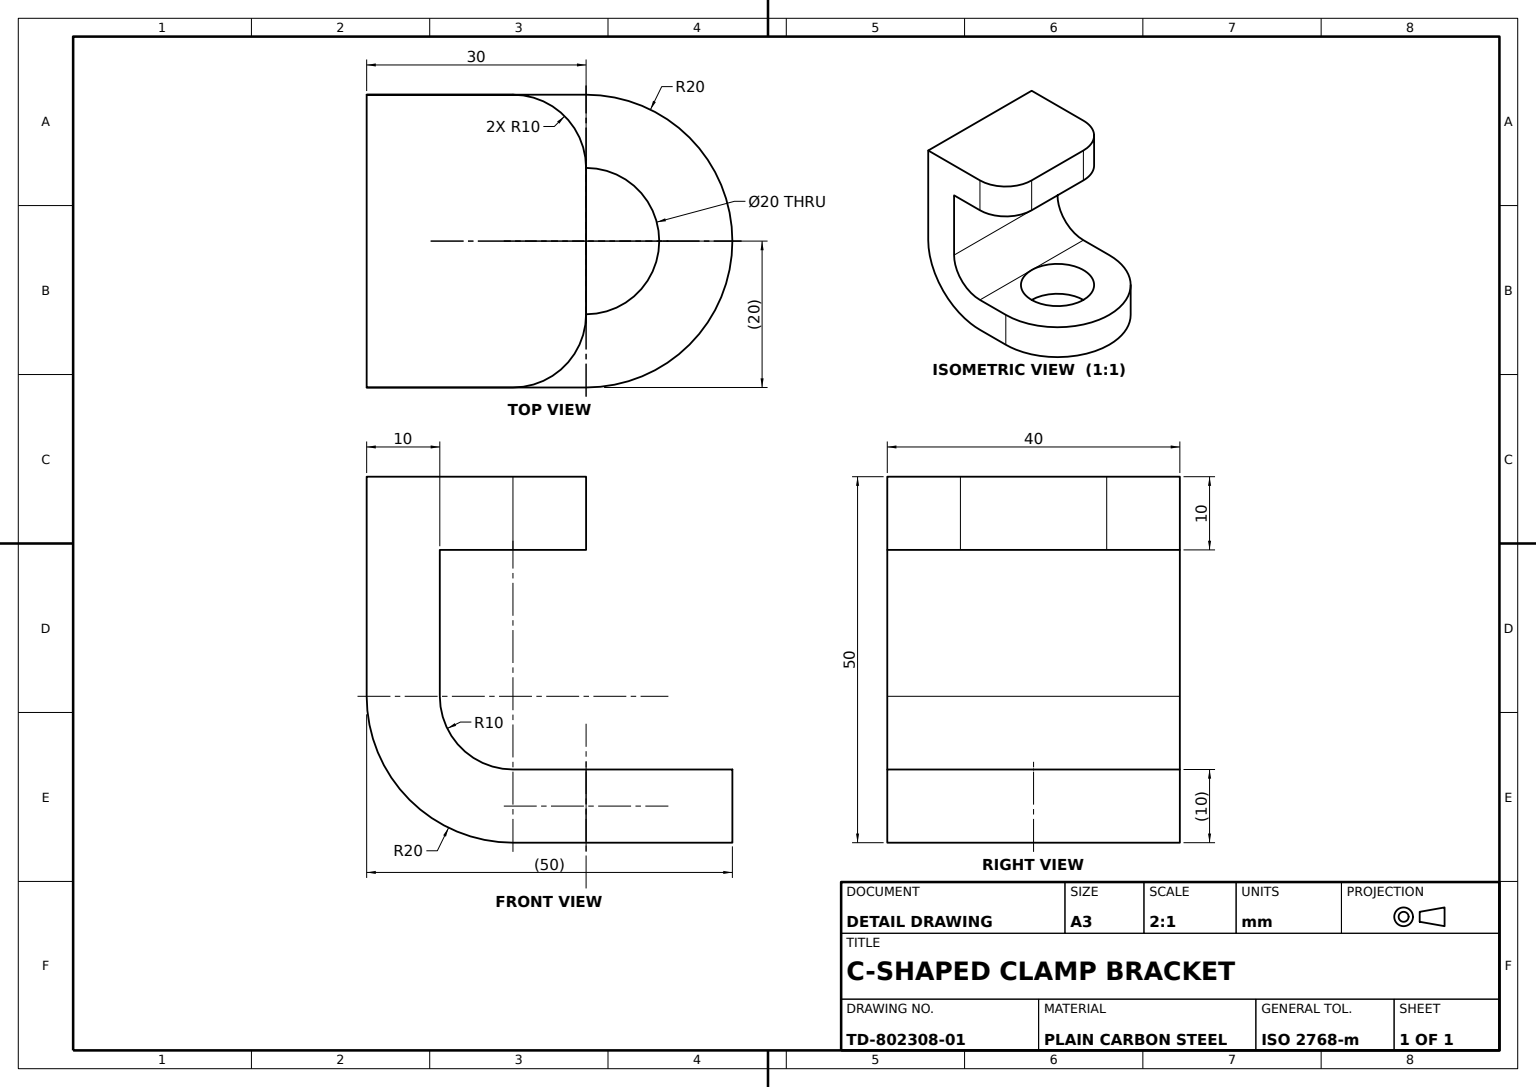
SolidWorks part; units mm, degrees
material "Plain Carbon Steel"
ref_plane "Front Plane" through (0, 0, 0) normal (0, 0, 1) x (1, 0, 0)
ref_plane "Top Plane" through (0, 0, 0) normal (0, 1, 0) x (1, 0, 0)
ref_plane "Right Plane" through (0, 0, 0) normal (1, 0, 0) x (0, 0, -1)
sketch "Bracket Profile Sketch" plane through (0, 0, 0) normal (0, 0, 1) x (1, 0, 0)
  line L0 (0, 20) -> (0, 50)
  line L1 (0, 50) -> (30, 50)
  line L2 (30, 50) -> (30, 40)
  line L3 (30, 40) -> (10, 40)
  line L4 (10, 40) -> (10, 20)
  line L5 (20, 10) -> (50, 10)
  line L6 (50, 10) -> (50, 0)
  line L7 (50, 0) -> (20, 0)
  arc A0 (10, 20) -> (20, 10) centre (20, 20) ccw
  arc A1 (0, 20) -> (20, 0) centre (20, 20) ccw
  point P13 (0, 0)
  dimension "D3" = 10
  dimension "D4" = 20
  dimension "D1" = 50
  dimension "D2" = 50
  dimension "D5" = 10
  dimension "D6" = 10
  dimension "D7" = 30
  dimension "D8" = 10
extrude "Bracket Body" add sketch "Bracket Profile Sketch" along normal mid plane 40
fillet "Edge Fillets R10" radius 10 2 edges at (30, 45, 20) (30, 45, -20)
sketch "Mounting Hole Sketch" plane through (0, 0, 0) normal (0, -1, 0) x (1, 0, 0)
  line L0 (50, 20) -> (50, -20) construction
  line L1 (20, 20) -> (50, 20) construction
  line L2 (20, 20) -> (50, 20)
  line L3 (50, 20) -> (50, -20)
  line L4 (20, -20) -> (50, -20) construction
  line L5 (20, -20) -> (50, -20)
  circle A0 centre (30, 0) radius 10
  circle A1 centre (30, 0) radius 20
  line M4 (50, -20) -> (50, 20)
  line M5 (50, 20) -> (20, 20)
  dimension "D1" = 40
  dimension "D2" = 20
extrude "Mounting Hole Cut" cut sketch "Mounting Hole Sketch" against normal up to surface (10 mm away) contours A1 L3 M5 | A1 L5 M4 | A0 up to face at (35, 10, 0)
